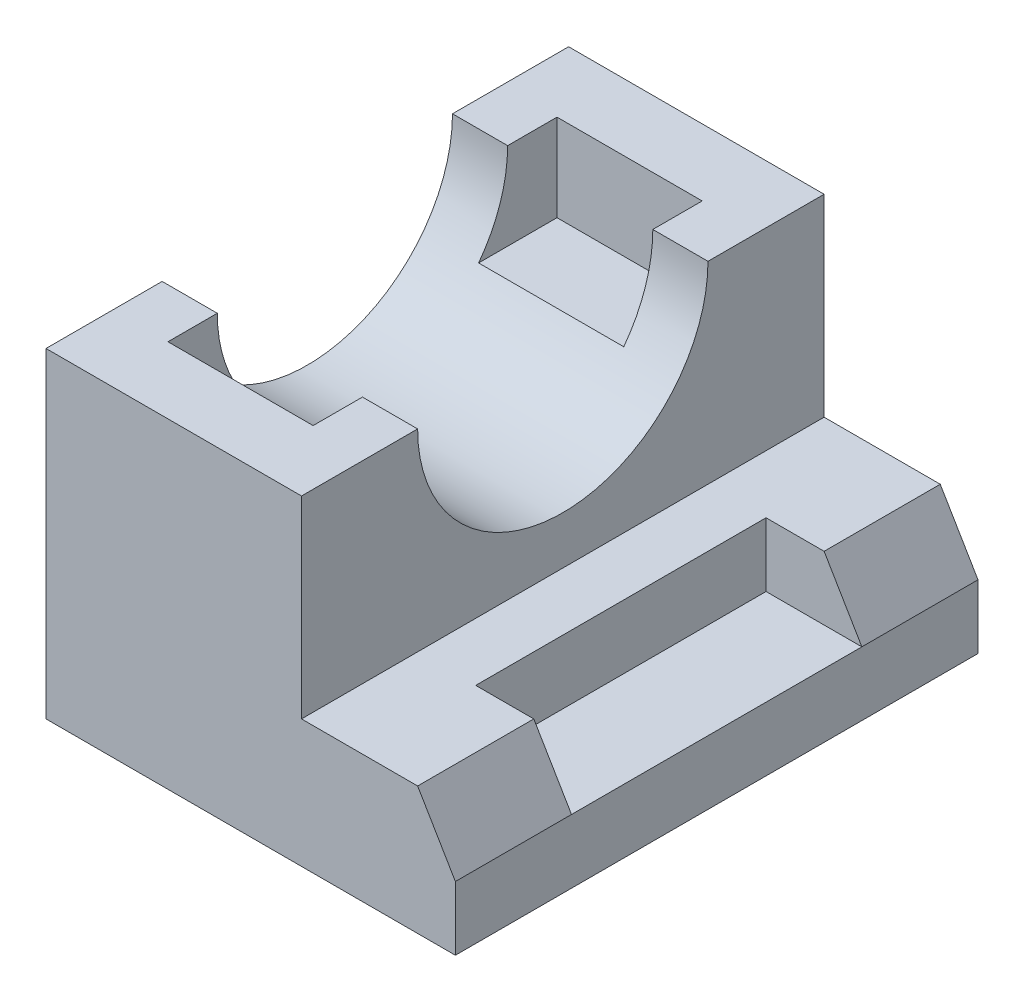
ISO-10303-21;
HEADER;
FILE_DESCRIPTION(('STEP AP214'),'2;1');
FILE_NAME('part.step','',(''),(''),'','','');
FILE_SCHEMA(('AUTOMOTIVE_DESIGN { 1 0 10303 214 1 1 1 1 }'));
ENDSEC;
DATA;
#1=APPLICATION_CONTEXT('core data for automotive mechanical design processes');
#2=APPLICATION_PROTOCOL_DEFINITION('international standard','automotive_design',2000,#1);
#3=PRODUCT_CONTEXT('',#1,'mechanical');
#4=PRODUCT('Part','Part','',(#3));
#5=PRODUCT_RELATED_PRODUCT_CATEGORY('part','',(#4));
#6=PRODUCT_DEFINITION_FORMATION('','',#4);
#7=PRODUCT_DEFINITION_CONTEXT('part definition',#1,'design');
#8=PRODUCT_DEFINITION('design','',#6,#7);
#9=PRODUCT_DEFINITION_SHAPE('','',#8);
#10=(LENGTH_UNIT() NAMED_UNIT(*) SI_UNIT(.MILLI.,.METRE.));
#11=(NAMED_UNIT(*) PLANE_ANGLE_UNIT() SI_UNIT($,.RADIAN.));
#12=(NAMED_UNIT(*) SI_UNIT($,.STERADIAN.) SOLID_ANGLE_UNIT());
#13=UNCERTAINTY_MEASURE_WITH_UNIT(LENGTH_MEASURE(1.E-05),#10,'distance_accuracy_value','');
#14=(GEOMETRIC_REPRESENTATION_CONTEXT(3) GLOBAL_UNCERTAINTY_ASSIGNED_CONTEXT((#13)) GLOBAL_UNIT_ASSIGNED_CONTEXT((#10,
#11,#12)) REPRESENTATION_CONTEXT('',''));
#15=CARTESIAN_POINT('',(0.,0.,0.));
#16=DIRECTION('',(0.,0.,1.));
#17=DIRECTION('',(1.,0.,0.));
#18=AXIS2_PLACEMENT_3D('',#15,#16,#17);
#19=CARTESIAN_POINT('',(57.0719754977029,33.7243491577335,45.));
#20=DIRECTION('',(0.860926528214316,0.50872931212664,0.));
#21=DIRECTION('',(-0.50872931212664,0.860926528214316,0.));
#22=AXIS2_PLACEMENT_3D('',#19,#20,#21);
#23=PLANE('',#22);
#24=DIRECTION('',(-0.50872931212664,0.860926528214316,0.));
#25=VECTOR('',#24,1.);
#26=CARTESIAN_POINT('',(57.071975497703,33.7243491577335,-25.));
#27=LINE('',#26,#25);
#28=CARTESIAN_POINT('',(70.5,11.,-25.));
#29=VERTEX_POINT('',#28);
#30=CARTESIAN_POINT('',(64.,22.,-25.));
#31=VERTEX_POINT('',#30);
#32=EDGE_CURVE('E251',#29,#31,#27,.T.);
#33=ORIENTED_EDGE('',*,*,#32,.F.);
#34=DIRECTION('',(0.,0.,-1.));
#35=VECTOR('',#34,1.);
#36=CARTESIAN_POINT('',(70.5,11.,45.));
#37=LINE('',#36,#35);
#38=CARTESIAN_POINT('',(70.5,11.,-45.));
#39=VERTEX_POINT('',#38);
#40=EDGE_CURVE('E312',#29,#39,#37,.T.);
#41=ORIENTED_EDGE('',*,*,#40,.T.);
#42=DIRECTION('',(0.50872931212664,-0.860926528214316,0.));
#43=VECTOR('',#42,1.);
#44=CARTESIAN_POINT('',(57.0719754977029,33.7243491577335,-45.));
#45=LINE('',#44,#43);
#46=CARTESIAN_POINT('',(64.,22.,-45.));
#47=VERTEX_POINT('',#46);
#48=EDGE_CURVE('E297',#47,#39,#45,.T.);
#49=ORIENTED_EDGE('',*,*,#48,.F.);
#50=DIRECTION('',(0.,0.,-1.));
#51=VECTOR('',#50,1.);
#52=CARTESIAN_POINT('',(64.,22.,45.));
#53=LINE('',#52,#51);
#54=EDGE_CURVE('E313',#31,#47,#53,.T.);
#55=ORIENTED_EDGE('',*,*,#54,.F.);
#56=EDGE_LOOP('',(#33,#41,#49,#55));
#57=FACE_BOUND('',#56,.T.);
#58=ADVANCED_FACE('F41',(#57),#23,.T.);
#59=CARTESIAN_POINT('',(0.,55.25,45.));
#60=DIRECTION('',(0.,-1.,0.));
#61=DIRECTION('',(1.,0.,0.));
#62=AXIS2_PLACEMENT_3D('',#59,#60,#61);
#63=PLANE('',#62);
#64=DIRECTION('',(-1.,0.,0.));
#65=VECTOR('',#64,1.);
#66=CARTESIAN_POINT('',(22.,55.25,-33.5));
#67=LINE('',#66,#65);
#68=CARTESIAN_POINT('',(34.5,55.25,-33.5));
#69=VERTEX_POINT('',#68);
#70=CARTESIAN_POINT('',(9.49999999999999,55.25,-33.5));
#71=VERTEX_POINT('',#70);
#72=EDGE_CURVE('E220',#69,#71,#67,.T.);
#73=ORIENTED_EDGE('',*,*,#72,.F.);
#74=DIRECTION('',(0.,0.,-1.));
#75=VECTOR('',#74,1.);
#76=CARTESIAN_POINT('',(34.5,55.25,-33.5));
#77=LINE('',#76,#75);
#78=CARTESIAN_POINT('',(34.5,55.25,-25.));
#79=VERTEX_POINT('',#78);
#80=EDGE_CURVE('E221',#79,#69,#77,.T.);
#81=ORIENTED_EDGE('',*,*,#80,.F.);
#82=DIRECTION('',(1.,0.,0.));
#83=VECTOR('',#82,1.);
#84=CARTESIAN_POINT('',(-1.,55.25,-25.));
#85=LINE('',#84,#83);
#86=CARTESIAN_POINT('',(44.,55.25,-25.));
#87=VERTEX_POINT('',#86);
#88=EDGE_CURVE('E256',#79,#87,#85,.T.);
#89=ORIENTED_EDGE('',*,*,#88,.T.);
#90=DIRECTION('',(0.,0.,-1.));
#91=VECTOR('',#90,1.);
#92=CARTESIAN_POINT('',(44.,55.25,45.));
#93=LINE('',#92,#91);
#94=CARTESIAN_POINT('',(44.,55.25,-45.));
#95=VERTEX_POINT('',#94);
#96=EDGE_CURVE('E286',#87,#95,#93,.T.);
#97=ORIENTED_EDGE('',*,*,#96,.T.);
#98=DIRECTION('',(-1.,0.,0.));
#99=VECTOR('',#98,1.);
#100=CARTESIAN_POINT('',(0.,55.25,-45.));
#101=LINE('',#100,#99);
#102=CARTESIAN_POINT('',(0.,55.25,-45.));
#103=VERTEX_POINT('',#102);
#104=EDGE_CURVE('E267',#95,#103,#101,.T.);
#105=ORIENTED_EDGE('',*,*,#104,.T.);
#106=DIRECTION('',(0.,0.,-1.));
#107=VECTOR('',#106,1.);
#108=CARTESIAN_POINT('',(0.,55.25,45.));
#109=LINE('',#108,#107);
#110=CARTESIAN_POINT('',(0.,55.25,-25.));
#111=VERTEX_POINT('',#110);
#112=EDGE_CURVE('E324',#111,#103,#109,.T.);
#113=ORIENTED_EDGE('',*,*,#112,.F.);
#114=CARTESIAN_POINT('',(9.49999999999999,55.25,-25.));
#115=VERTEX_POINT('',#114);
#116=EDGE_CURVE('E262',#111,#115,#85,.T.);
#117=ORIENTED_EDGE('',*,*,#116,.T.);
#118=DIRECTION('',(0.,0.,1.));
#119=VECTOR('',#118,1.);
#120=CARTESIAN_POINT('',(9.49999999999999,55.25,-18.5));
#121=LINE('',#120,#119);
#122=EDGE_CURVE('E225',#71,#115,#121,.T.);
#123=ORIENTED_EDGE('',*,*,#122,.F.);
#124=EDGE_LOOP('',(#73,#81,#89,#97,#105,#113,#117,#123));
#125=FACE_BOUND('',#124,.T.);
#126=ADVANCED_FACE('F363',(#125),#63,.F.);
#127=DIRECTION('',(1.,0.,0.));
#128=VECTOR('',#127,1.);
#129=CARTESIAN_POINT('',(22.,55.25,33.5));
#130=LINE('',#129,#128);
#131=CARTESIAN_POINT('',(9.49999999999999,55.25,33.5));
#132=VERTEX_POINT('',#131);
#133=CARTESIAN_POINT('',(34.5,55.25,33.5));
#134=VERTEX_POINT('',#133);
#135=EDGE_CURVE('E207',#132,#134,#130,.T.);
#136=ORIENTED_EDGE('',*,*,#135,.F.);
#137=DIRECTION('',(0.,0.,1.));
#138=VECTOR('',#137,1.);
#139=CARTESIAN_POINT('',(9.49999999999999,55.25,18.5));
#140=LINE('',#139,#138);
#141=CARTESIAN_POINT('',(9.49999999999999,55.25,25.));
#142=VERTEX_POINT('',#141);
#143=EDGE_CURVE('E196',#142,#132,#140,.T.);
#144=ORIENTED_EDGE('',*,*,#143,.F.);
#145=DIRECTION('',(1.,0.,0.));
#146=VECTOR('',#145,1.);
#147=CARTESIAN_POINT('',(-1.,55.25,25.));
#148=LINE('',#147,#146);
#149=CARTESIAN_POINT('',(0.,55.25,25.));
#150=VERTEX_POINT('',#149);
#151=EDGE_CURVE('E259',#150,#142,#148,.T.);
#152=ORIENTED_EDGE('',*,*,#151,.F.);
#153=CARTESIAN_POINT('',(0.,55.25,45.));
#154=VERTEX_POINT('',#153);
#155=EDGE_CURVE('E326',#154,#150,#109,.T.);
#156=ORIENTED_EDGE('',*,*,#155,.F.);
#157=DIRECTION('',(-1.,0.,0.));
#158=VECTOR('',#157,1.);
#159=CARTESIAN_POINT('',(0.,55.25,45.));
#160=LINE('',#159,#158);
#161=CARTESIAN_POINT('',(44.,55.25,45.));
#162=VERTEX_POINT('',#161);
#163=EDGE_CURVE('E269',#162,#154,#160,.T.);
#164=ORIENTED_EDGE('',*,*,#163,.F.);
#165=CARTESIAN_POINT('',(44.,55.25,25.));
#166=VERTEX_POINT('',#165);
#167=EDGE_CURVE('E308',#162,#166,#93,.T.);
#168=ORIENTED_EDGE('',*,*,#167,.T.);
#169=CARTESIAN_POINT('',(34.5,55.25,25.));
#170=VERTEX_POINT('',#169);
#171=EDGE_CURVE('E263',#170,#166,#148,.T.);
#172=ORIENTED_EDGE('',*,*,#171,.F.);
#173=DIRECTION('',(0.,0.,-1.));
#174=VECTOR('',#173,1.);
#175=CARTESIAN_POINT('',(34.5,55.25,33.5));
#176=LINE('',#175,#174);
#177=EDGE_CURVE('E195',#134,#170,#176,.T.);
#178=ORIENTED_EDGE('',*,*,#177,.F.);
#179=EDGE_LOOP('',(#136,#144,#152,#156,#164,#168,#172,#178));
#180=FACE_BOUND('',#179,.T.);
#181=ADVANCED_FACE('F43',(#180),#63,.F.);
#182=CARTESIAN_POINT('',(0.,0.,45.));
#183=DIRECTION('',(1.,0.,0.));
#184=DIRECTION('',(0.,1.,0.));
#185=AXIS2_PLACEMENT_3D('',#182,#183,#184);
#186=PLANE('',#185);
#187=ORIENTED_EDGE('',*,*,#155,.T.);
#188=CARTESIAN_POINT('',(0.,55.25,0.));
#189=DIRECTION('',(1.,0.,0.));
#190=DIRECTION('',(0.,1.,0.));
#191=AXIS2_PLACEMENT_3D('',#188,#189,#190);
#192=CIRCLE('',#191,25.);
#193=EDGE_CURVE('E265',#150,#111,#192,.T.);
#194=ORIENTED_EDGE('',*,*,#193,.T.);
#195=ORIENTED_EDGE('',*,*,#112,.T.);
#196=DIRECTION('',(0.,-1.,0.));
#197=VECTOR('',#196,1.);
#198=CARTESIAN_POINT('',(0.,0.,-45.));
#199=LINE('',#198,#197);
#200=CARTESIAN_POINT('',(0.,0.,-45.));
#201=VERTEX_POINT('',#200);
#202=EDGE_CURVE('E292',#103,#201,#199,.T.);
#203=ORIENTED_EDGE('',*,*,#202,.T.);
#204=DIRECTION('',(0.,0.,-1.));
#205=VECTOR('',#204,1.);
#206=CARTESIAN_POINT('',(0.,0.,45.));
#207=LINE('',#206,#205);
#208=CARTESIAN_POINT('',(0.,0.,45.));
#209=VERTEX_POINT('',#208);
#210=EDGE_CURVE('E325',#209,#201,#207,.T.);
#211=ORIENTED_EDGE('',*,*,#210,.F.);
#212=DIRECTION('',(0.,-1.,0.));
#213=VECTOR('',#212,1.);
#214=CARTESIAN_POINT('',(0.,0.,45.));
#215=LINE('',#214,#213);
#216=EDGE_CURVE('E272',#154,#209,#215,.T.);
#217=ORIENTED_EDGE('',*,*,#216,.F.);
#218=EDGE_LOOP('',(#187,#194,#195,#203,#211,#217));
#219=FACE_BOUND('',#218,.T.);
#220=ADVANCED_FACE('F376',(#219),#186,.F.);
#221=CARTESIAN_POINT('',(0.,0.,45.));
#222=DIRECTION('',(0.,1.,0.));
#223=DIRECTION('',(0.,0.,1.));
#224=AXIS2_PLACEMENT_3D('',#221,#222,#223);
#225=PLANE('',#224);
#226=DIRECTION('',(1.,0.,0.));
#227=VECTOR('',#226,1.);
#228=CARTESIAN_POINT('',(0.,0.,-45.));
#229=LINE('',#228,#227);
#230=CARTESIAN_POINT('',(70.5,0.,-45.));
#231=VERTEX_POINT('',#230);
#232=EDGE_CURVE('E291',#201,#231,#229,.T.);
#233=ORIENTED_EDGE('',*,*,#232,.T.);
#234=DIRECTION('',(0.,0.,-1.));
#235=VECTOR('',#234,1.);
#236=CARTESIAN_POINT('',(70.5,0.,45.));
#237=LINE('',#236,#235);
#238=CARTESIAN_POINT('',(70.5,0.,45.));
#239=VERTEX_POINT('',#238);
#240=EDGE_CURVE('E317',#239,#231,#237,.T.);
#241=ORIENTED_EDGE('',*,*,#240,.F.);
#242=DIRECTION('',(1.,0.,0.));
#243=VECTOR('',#242,1.);
#244=CARTESIAN_POINT('',(0.,0.,45.));
#245=LINE('',#244,#243);
#246=EDGE_CURVE('E277',#209,#239,#245,.T.);
#247=ORIENTED_EDGE('',*,*,#246,.F.);
#248=ORIENTED_EDGE('',*,*,#210,.T.);
#249=EDGE_LOOP('',(#233,#241,#247,#248));
#250=FACE_BOUND('',#249,.T.);
#251=ADVANCED_FACE('F384',(#250),#225,.F.);
#252=CARTESIAN_POINT('',(70.5,0.,45.));
#253=DIRECTION('',(-1.,0.,0.));
#254=DIRECTION('',(0.,0.,1.));
#255=AXIS2_PLACEMENT_3D('',#252,#253,#254);
#256=PLANE('',#255);
#257=DIRECTION('',(0.,1.,0.));
#258=VECTOR('',#257,1.);
#259=CARTESIAN_POINT('',(70.5,0.,-45.));
#260=LINE('',#259,#258);
#261=EDGE_CURVE('E293',#231,#39,#260,.T.);
#262=ORIENTED_EDGE('',*,*,#261,.T.);
#263=ORIENTED_EDGE('',*,*,#40,.F.);
#264=DIRECTION('',(0.,0.,-1.));
#265=VECTOR('',#264,1.);
#266=CARTESIAN_POINT('',(70.5,11.,-25.));
#267=LINE('',#266,#265);
#268=CARTESIAN_POINT('',(70.5,11.,25.));
#269=VERTEX_POINT('',#268);
#270=EDGE_CURVE('E241',#269,#29,#267,.T.);
#271=ORIENTED_EDGE('',*,*,#270,.F.);
#272=CARTESIAN_POINT('',(70.5,11.,45.));
#273=VERTEX_POINT('',#272);
#274=EDGE_CURVE('E316',#273,#269,#37,.T.);
#275=ORIENTED_EDGE('',*,*,#274,.F.);
#276=DIRECTION('',(0.,1.,0.));
#277=VECTOR('',#276,1.);
#278=CARTESIAN_POINT('',(70.5,0.,45.));
#279=LINE('',#278,#277);
#280=EDGE_CURVE('E279',#239,#273,#279,.T.);
#281=ORIENTED_EDGE('',*,*,#280,.F.);
#282=ORIENTED_EDGE('',*,*,#240,.T.);
#283=EDGE_LOOP('',(#262,#263,#271,#275,#281,#282));
#284=FACE_BOUND('',#283,.T.);
#285=ADVANCED_FACE('F386',(#284),#256,.F.);
#286=DIRECTION('',(0.50872931212664,-0.860926528214316,0.));
#287=VECTOR('',#286,1.);
#288=CARTESIAN_POINT('',(57.0719754977029,33.7243491577335,25.));
#289=LINE('',#288,#287);
#290=CARTESIAN_POINT('',(64.,22.,25.));
#291=VERTEX_POINT('',#290);
#292=EDGE_CURVE('E247',#291,#269,#289,.T.);
#293=ORIENTED_EDGE('',*,*,#292,.F.);
#294=CARTESIAN_POINT('',(64.,22.,45.));
#295=VERTEX_POINT('',#294);
#296=EDGE_CURVE('E315',#295,#291,#53,.T.);
#297=ORIENTED_EDGE('',*,*,#296,.F.);
#298=DIRECTION('',(0.50872931212664,-0.860926528214316,0.));
#299=VECTOR('',#298,1.);
#300=CARTESIAN_POINT('',(57.0719754977029,33.7243491577335,45.));
#301=LINE('',#300,#299);
#302=EDGE_CURVE('E278',#295,#273,#301,.T.);
#303=ORIENTED_EDGE('',*,*,#302,.T.);
#304=ORIENTED_EDGE('',*,*,#274,.T.);
#305=EDGE_LOOP('',(#293,#297,#303,#304));
#306=FACE_BOUND('',#305,.T.);
#307=ADVANCED_FACE('F408',(#306),#23,.T.);
#308=CARTESIAN_POINT('',(0.,22.,45.));
#309=DIRECTION('',(0.,1.,0.));
#310=DIRECTION('',(0.,0.,1.));
#311=AXIS2_PLACEMENT_3D('',#308,#309,#310);
#312=PLANE('',#311);
#313=DIRECTION('',(-1.,0.,0.));
#314=VECTOR('',#313,1.);
#315=CARTESIAN_POINT('',(0.,22.,-25.));
#316=LINE('',#315,#314);
#317=CARTESIAN_POINT('',(54.,22.,-25.));
#318=VERTEX_POINT('',#317);
#319=EDGE_CURVE('E328',#31,#318,#316,.T.);
#320=ORIENTED_EDGE('',*,*,#319,.F.);
#321=ORIENTED_EDGE('',*,*,#54,.T.);
#322=DIRECTION('',(1.,0.,0.));
#323=VECTOR('',#322,1.);
#324=CARTESIAN_POINT('',(0.,22.,-45.));
#325=LINE('',#324,#323);
#326=CARTESIAN_POINT('',(44.,22.,-45.));
#327=VERTEX_POINT('',#326);
#328=EDGE_CURVE('E303',#327,#47,#325,.T.);
#329=ORIENTED_EDGE('',*,*,#328,.F.);
#330=DIRECTION('',(0.,0.,-1.));
#331=VECTOR('',#330,1.);
#332=CARTESIAN_POINT('',(44.,22.,45.));
#333=LINE('',#332,#331);
#334=CARTESIAN_POINT('',(44.,22.,45.));
#335=VERTEX_POINT('',#334);
#336=EDGE_CURVE('E310',#335,#327,#333,.T.);
#337=ORIENTED_EDGE('',*,*,#336,.F.);
#338=DIRECTION('',(1.,0.,0.));
#339=VECTOR('',#338,1.);
#340=CARTESIAN_POINT('',(0.,22.,45.));
#341=LINE('',#340,#339);
#342=EDGE_CURVE('E282',#335,#295,#341,.T.);
#343=ORIENTED_EDGE('',*,*,#342,.T.);
#344=ORIENTED_EDGE('',*,*,#296,.T.);
#345=DIRECTION('',(1.,0.,0.));
#346=VECTOR('',#345,1.);
#347=CARTESIAN_POINT('',(70.5,22.,25.));
#348=LINE('',#347,#346);
#349=CARTESIAN_POINT('',(54.,22.,25.));
#350=VERTEX_POINT('',#349);
#351=EDGE_CURVE('E232',#350,#291,#348,.T.);
#352=ORIENTED_EDGE('',*,*,#351,.F.);
#353=DIRECTION('',(0.,0.,1.));
#354=VECTOR('',#353,1.);
#355=CARTESIAN_POINT('',(54.,22.,25.));
#356=LINE('',#355,#354);
#357=EDGE_CURVE('E213',#318,#350,#356,.T.);
#358=ORIENTED_EDGE('',*,*,#357,.F.);
#359=EDGE_LOOP('',(#320,#321,#329,#337,#343,#344,#352,#358));
#360=FACE_BOUND('',#359,.T.);
#361=ADVANCED_FACE('F399',(#360),#312,.T.);
#362=CARTESIAN_POINT('',(44.,0.,45.));
#363=DIRECTION('',(-1.,0.,0.));
#364=DIRECTION('',(0.,0.,1.));
#365=AXIS2_PLACEMENT_3D('',#362,#363,#364);
#366=PLANE('',#365);
#367=ORIENTED_EDGE('',*,*,#96,.F.);
#368=CARTESIAN_POINT('',(44.,55.25,0.));
#369=DIRECTION('',(1.,0.,0.));
#370=DIRECTION('',(0.,0.,-1.));
#371=AXIS2_PLACEMENT_3D('',#368,#369,#370);
#372=CIRCLE('',#371,25.);
#373=EDGE_CURVE('E254',#166,#87,#372,.T.);
#374=ORIENTED_EDGE('',*,*,#373,.F.);
#375=ORIENTED_EDGE('',*,*,#167,.F.);
#376=DIRECTION('',(0.,1.,0.));
#377=VECTOR('',#376,1.);
#378=CARTESIAN_POINT('',(44.,0.,45.));
#379=LINE('',#378,#377);
#380=EDGE_CURVE('E288',#335,#162,#379,.T.);
#381=ORIENTED_EDGE('',*,*,#380,.F.);
#382=ORIENTED_EDGE('',*,*,#336,.T.);
#383=DIRECTION('',(0.,1.,0.));
#384=VECTOR('',#383,1.);
#385=CARTESIAN_POINT('',(44.,0.,-45.));
#386=LINE('',#385,#384);
#387=EDGE_CURVE('E273',#327,#95,#386,.T.);
#388=ORIENTED_EDGE('',*,*,#387,.T.);
#389=EDGE_LOOP('',(#367,#374,#375,#381,#382,#388));
#390=FACE_BOUND('',#389,.T.);
#391=ADVANCED_FACE('F354',(#390),#366,.F.);
#392=CARTESIAN_POINT('',(0.,0.,45.));
#393=DIRECTION('',(0.,0.,1.));
#394=DIRECTION('',(1.,0.,0.));
#395=AXIS2_PLACEMENT_3D('',#392,#393,#394);
#396=PLANE('',#395);
#397=ORIENTED_EDGE('',*,*,#163,.T.);
#398=ORIENTED_EDGE('',*,*,#216,.T.);
#399=ORIENTED_EDGE('',*,*,#246,.T.);
#400=ORIENTED_EDGE('',*,*,#280,.T.);
#401=ORIENTED_EDGE('',*,*,#302,.F.);
#402=ORIENTED_EDGE('',*,*,#342,.F.);
#403=ORIENTED_EDGE('',*,*,#380,.T.);
#404=EDGE_LOOP('',(#397,#398,#399,#400,#401,#402,#403));
#405=FACE_BOUND('',#404,.T.);
#406=ADVANCED_FACE('F394',(#405),#396,.T.);
#407=CARTESIAN_POINT('',(0.,0.,-45.));
#408=DIRECTION('',(0.,0.,1.));
#409=DIRECTION('',(1.,0.,0.));
#410=AXIS2_PLACEMENT_3D('',#407,#408,#409);
#411=PLANE('',#410);
#412=ORIENTED_EDGE('',*,*,#104,.F.);
#413=ORIENTED_EDGE('',*,*,#387,.F.);
#414=ORIENTED_EDGE('',*,*,#328,.T.);
#415=ORIENTED_EDGE('',*,*,#48,.T.);
#416=ORIENTED_EDGE('',*,*,#261,.F.);
#417=ORIENTED_EDGE('',*,*,#232,.F.);
#418=ORIENTED_EDGE('',*,*,#202,.F.);
#419=EDGE_LOOP('',(#412,#413,#414,#415,#416,#417,#418));
#420=FACE_BOUND('',#419,.T.);
#421=ADVANCED_FACE('F379',(#420),#411,.F.);
#422=CARTESIAN_POINT('',(-1.,55.25,0.));
#423=DIRECTION('',(1.,0.,0.));
#424=DIRECTION('',(0.,0.,-1.));
#425=AXIS2_PLACEMENT_3D('',#422,#423,#424);
#426=CYLINDRICAL_SURFACE('',#425,25.);
#427=ORIENTED_EDGE('',*,*,#151,.T.);
#428=CARTESIAN_POINT('',(9.49999999999999,55.25,0.));
#429=DIRECTION('',(-1.,0.,0.));
#430=DIRECTION('',(0.,-1.,0.));
#431=AXIS2_PLACEMENT_3D('',#428,#429,#430);
#432=CIRCLE('',#431,25.);
#433=CARTESIAN_POINT('',(9.49999999999999,40.25,20.));
#434=VERTEX_POINT('',#433);
#435=EDGE_CURVE('E11',#142,#434,#432,.F.);
#436=ORIENTED_EDGE('',*,*,#435,.T.);
#437=DIRECTION('',(1.,0.,0.));
#438=VECTOR('',#437,1.);
#439=CARTESIAN_POINT('',(-0.999999999999993,40.25,20.));
#440=LINE('',#439,#438);
#441=CARTESIAN_POINT('',(34.5,40.25,20.));
#442=VERTEX_POINT('',#441);
#443=EDGE_CURVE('E189',#442,#434,#440,.F.);
#444=ORIENTED_EDGE('',*,*,#443,.F.);
#445=CARTESIAN_POINT('',(34.5,55.25,0.));
#446=DIRECTION('',(1.,0.,0.));
#447=DIRECTION('',(0.,1.,0.));
#448=AXIS2_PLACEMENT_3D('',#445,#446,#447);
#449=CIRCLE('',#448,25.);
#450=EDGE_CURVE('E47',#442,#170,#449,.F.);
#451=ORIENTED_EDGE('',*,*,#450,.T.);
#452=ORIENTED_EDGE('',*,*,#171,.T.);
#453=ORIENTED_EDGE('',*,*,#373,.T.);
#454=ORIENTED_EDGE('',*,*,#88,.F.);
#455=CARTESIAN_POINT('',(34.5,55.25,0.));
#456=DIRECTION('',(1.,0.,0.));
#457=DIRECTION('',(0.,1.,0.));
#458=AXIS2_PLACEMENT_3D('',#455,#456,#457);
#459=CIRCLE('',#458,25.);
#460=CARTESIAN_POINT('',(34.5,40.25,-20.));
#461=VERTEX_POINT('',#460);
#462=EDGE_CURVE('E337',#79,#461,#459,.F.);
#463=ORIENTED_EDGE('',*,*,#462,.T.);
#464=DIRECTION('',(1.,0.,0.));
#465=VECTOR('',#464,1.);
#466=CARTESIAN_POINT('',(-0.999999999999993,40.25,-20.));
#467=LINE('',#466,#465);
#468=CARTESIAN_POINT('',(9.49999999999999,40.25,-20.));
#469=VERTEX_POINT('',#468);
#470=EDGE_CURVE('E335',#461,#469,#467,.F.);
#471=ORIENTED_EDGE('',*,*,#470,.T.);
#472=CARTESIAN_POINT('',(9.49999999999999,55.25,0.));
#473=DIRECTION('',(-1.,0.,0.));
#474=DIRECTION('',(0.,-1.,0.));
#475=AXIS2_PLACEMENT_3D('',#472,#473,#474);
#476=CIRCLE('',#475,25.);
#477=EDGE_CURVE('E333',#469,#115,#476,.F.);
#478=ORIENTED_EDGE('',*,*,#477,.T.);
#479=ORIENTED_EDGE('',*,*,#116,.F.);
#480=ORIENTED_EDGE('',*,*,#193,.F.);
#481=EDGE_LOOP('',(#427,#436,#444,#451,#452,#453,#454,#463,#471,#478,#479,#480));
#482=FACE_BOUND('',#481,.T.);
#483=ADVANCED_FACE('F344',(#482),#426,.F.);
#484=CARTESIAN_POINT('',(54.,11.,-25.));
#485=DIRECTION('',(0.,0.,-1.));
#486=DIRECTION('',(-1.,0.,0.));
#487=AXIS2_PLACEMENT_3D('',#484,#485,#486);
#488=PLANE('',#487);
#489=ORIENTED_EDGE('',*,*,#32,.T.);
#490=ORIENTED_EDGE('',*,*,#319,.T.);
#491=DIRECTION('',(0.,1.,0.));
#492=VECTOR('',#491,1.);
#493=CARTESIAN_POINT('',(54.,11.,-25.));
#494=LINE('',#493,#492);
#495=CARTESIAN_POINT('',(54.,11.,-25.));
#496=VERTEX_POINT('',#495);
#497=EDGE_CURVE('E243',#496,#318,#494,.T.);
#498=ORIENTED_EDGE('',*,*,#497,.F.);
#499=DIRECTION('',(-1.,0.,0.));
#500=VECTOR('',#499,1.);
#501=CARTESIAN_POINT('',(54.,11.,-25.));
#502=LINE('',#501,#500);
#503=EDGE_CURVE('E233',#29,#496,#502,.T.);
#504=ORIENTED_EDGE('',*,*,#503,.F.);
#505=EDGE_LOOP('',(#489,#490,#498,#504));
#506=FACE_BOUND('',#505,.T.);
#507=ADVANCED_FACE('F420',(#506),#488,.F.);
#508=CARTESIAN_POINT('',(70.5,11.,25.));
#509=DIRECTION('',(0.,0.,1.));
#510=DIRECTION('',(1.,0.,0.));
#511=AXIS2_PLACEMENT_3D('',#508,#509,#510);
#512=PLANE('',#511);
#513=ORIENTED_EDGE('',*,*,#292,.T.);
#514=DIRECTION('',(1.,0.,0.));
#515=VECTOR('',#514,1.);
#516=CARTESIAN_POINT('',(70.5,11.,25.));
#517=LINE('',#516,#515);
#518=CARTESIAN_POINT('',(54.,11.,25.));
#519=VERTEX_POINT('',#518);
#520=EDGE_CURVE('E236',#519,#269,#517,.T.);
#521=ORIENTED_EDGE('',*,*,#520,.F.);
#522=DIRECTION('',(0.,1.,0.));
#523=VECTOR('',#522,1.);
#524=CARTESIAN_POINT('',(54.,11.,25.));
#525=LINE('',#524,#523);
#526=EDGE_CURVE('E246',#519,#350,#525,.T.);
#527=ORIENTED_EDGE('',*,*,#526,.T.);
#528=ORIENTED_EDGE('',*,*,#351,.T.);
#529=EDGE_LOOP('',(#513,#521,#527,#528));
#530=FACE_BOUND('',#529,.T.);
#531=ADVANCED_FACE('F415',(#530),#512,.F.);
#532=CARTESIAN_POINT('',(54.,11.,25.));
#533=DIRECTION('',(-1.,0.,0.));
#534=DIRECTION('',(0.,0.,1.));
#535=AXIS2_PLACEMENT_3D('',#532,#533,#534);
#536=PLANE('',#535);
#537=ORIENTED_EDGE('',*,*,#357,.T.);
#538=ORIENTED_EDGE('',*,*,#526,.F.);
#539=DIRECTION('',(0.,0.,1.));
#540=VECTOR('',#539,1.);
#541=CARTESIAN_POINT('',(54.,11.,25.));
#542=LINE('',#541,#540);
#543=EDGE_CURVE('E234',#496,#519,#542,.T.);
#544=ORIENTED_EDGE('',*,*,#543,.F.);
#545=ORIENTED_EDGE('',*,*,#497,.T.);
#546=EDGE_LOOP('',(#537,#538,#544,#545));
#547=FACE_BOUND('',#546,.T.);
#548=ADVANCED_FACE('F418',(#547),#536,.F.);
#549=CARTESIAN_POINT('',(0.,11.,0.));
#550=DIRECTION('',(0.,-1.,0.));
#551=DIRECTION('',(0.,0.,-1.));
#552=AXIS2_PLACEMENT_3D('',#549,#550,#551);
#553=PLANE('',#552);
#554=ORIENTED_EDGE('',*,*,#503,.T.);
#555=ORIENTED_EDGE('',*,*,#543,.T.);
#556=ORIENTED_EDGE('',*,*,#520,.T.);
#557=ORIENTED_EDGE('',*,*,#270,.T.);
#558=EDGE_LOOP('',(#554,#555,#556,#557));
#559=FACE_BOUND('',#558,.T.);
#560=ADVANCED_FACE('F411',(#559),#553,.F.);
#561=CARTESIAN_POINT('',(34.5,40.25,-33.5));
#562=DIRECTION('',(1.,0.,0.));
#563=DIRECTION('',(0.,1.,0.));
#564=AXIS2_PLACEMENT_3D('',#561,#562,#563);
#565=PLANE('',#564);
#566=ORIENTED_EDGE('',*,*,#80,.T.);
#567=DIRECTION('',(0.,1.,0.));
#568=VECTOR('',#567,1.);
#569=CARTESIAN_POINT('',(34.5,40.25,-33.5));
#570=LINE('',#569,#568);
#571=CARTESIAN_POINT('',(34.5,40.25,-33.5));
#572=VERTEX_POINT('',#571);
#573=EDGE_CURVE('E209',#572,#69,#570,.T.);
#574=ORIENTED_EDGE('',*,*,#573,.F.);
#575=DIRECTION('',(0.,0.,-1.));
#576=VECTOR('',#575,1.);
#577=CARTESIAN_POINT('',(34.5,40.25,-33.5));
#578=LINE('',#577,#576);
#579=EDGE_CURVE('E218',#461,#572,#578,.T.);
#580=ORIENTED_EDGE('',*,*,#579,.F.);
#581=ORIENTED_EDGE('',*,*,#462,.F.);
#582=EDGE_LOOP('',(#566,#574,#580,#581));
#583=FACE_BOUND('',#582,.T.);
#584=ADVANCED_FACE('F364',(#583),#565,.F.);
#585=CARTESIAN_POINT('',(9.49999999999999,40.25,-18.5));
#586=DIRECTION('',(-1.,0.,0.));
#587=DIRECTION('',(0.,-1.,0.));
#588=AXIS2_PLACEMENT_3D('',#585,#586,#587);
#589=PLANE('',#588);
#590=DIRECTION('',(0.,0.,1.));
#591=VECTOR('',#590,1.);
#592=CARTESIAN_POINT('',(9.49999999999999,40.25,-18.5));
#593=LINE('',#592,#591);
#594=CARTESIAN_POINT('',(9.49999999999999,40.25,-33.5));
#595=VERTEX_POINT('',#594);
#596=EDGE_CURVE('E63',#595,#469,#593,.T.);
#597=ORIENTED_EDGE('',*,*,#596,.F.);
#598=DIRECTION('',(0.,1.,0.));
#599=VECTOR('',#598,1.);
#600=CARTESIAN_POINT('',(9.49999999999999,40.25,-33.5));
#601=LINE('',#600,#599);
#602=EDGE_CURVE('E222',#595,#71,#601,.T.);
#603=ORIENTED_EDGE('',*,*,#602,.T.);
#604=ORIENTED_EDGE('',*,*,#122,.T.);
#605=ORIENTED_EDGE('',*,*,#477,.F.);
#606=EDGE_LOOP('',(#597,#603,#604,#605));
#607=FACE_BOUND('',#606,.T.);
#608=ADVANCED_FACE('F467',(#607),#589,.F.);
#609=CARTESIAN_POINT('',(0.,40.25,0.));
#610=DIRECTION('',(0.,-1.,0.));
#611=DIRECTION('',(1.,0.,0.));
#612=AXIS2_PLACEMENT_3D('',#609,#610,#611);
#613=PLANE('',#612);
#614=ORIENTED_EDGE('',*,*,#579,.T.);
#615=DIRECTION('',(-1.,0.,0.));
#616=VECTOR('',#615,1.);
#617=CARTESIAN_POINT('',(9.49999999999999,40.25,-33.5));
#618=LINE('',#617,#616);
#619=EDGE_CURVE('E214',#572,#595,#618,.T.);
#620=ORIENTED_EDGE('',*,*,#619,.T.);
#621=ORIENTED_EDGE('',*,*,#596,.T.);
#622=ORIENTED_EDGE('',*,*,#470,.F.);
#623=EDGE_LOOP('',(#614,#620,#621,#622));
#624=FACE_BOUND('',#623,.T.);
#625=ADVANCED_FACE('F367',(#624),#613,.F.);
#626=CARTESIAN_POINT('',(22.,40.25,-33.5));
#627=DIRECTION('',(0.,0.,-1.));
#628=DIRECTION('',(-1.,0.,0.));
#629=AXIS2_PLACEMENT_3D('',#626,#627,#628);
#630=PLANE('',#629);
#631=ORIENTED_EDGE('',*,*,#72,.T.);
#632=ORIENTED_EDGE('',*,*,#602,.F.);
#633=ORIENTED_EDGE('',*,*,#619,.F.);
#634=ORIENTED_EDGE('',*,*,#573,.T.);
#635=EDGE_LOOP('',(#631,#632,#633,#634));
#636=FACE_BOUND('',#635,.T.);
#637=ADVANCED_FACE('F369',(#636),#630,.F.);
#638=CARTESIAN_POINT('',(9.49999999999999,40.25,18.5));
#639=DIRECTION('',(-1.,0.,0.));
#640=DIRECTION('',(0.,-1.,0.));
#641=AXIS2_PLACEMENT_3D('',#638,#639,#640);
#642=PLANE('',#641);
#643=ORIENTED_EDGE('',*,*,#143,.T.);
#644=DIRECTION('',(0.,1.,0.));
#645=VECTOR('',#644,1.);
#646=CARTESIAN_POINT('',(9.49999999999999,40.25,33.5));
#647=LINE('',#646,#645);
#648=CARTESIAN_POINT('',(9.49999999999999,40.25,33.5));
#649=VERTEX_POINT('',#648);
#650=EDGE_CURVE('E192',#649,#132,#647,.T.);
#651=ORIENTED_EDGE('',*,*,#650,.F.);
#652=DIRECTION('',(0.,0.,1.));
#653=VECTOR('',#652,1.);
#654=CARTESIAN_POINT('',(9.49999999999999,40.25,18.5));
#655=LINE('',#654,#653);
#656=EDGE_CURVE('E181',#434,#649,#655,.T.);
#657=ORIENTED_EDGE('',*,*,#656,.F.);
#658=ORIENTED_EDGE('',*,*,#435,.F.);
#659=EDGE_LOOP('',(#643,#651,#657,#658));
#660=FACE_BOUND('',#659,.T.);
#661=ADVANCED_FACE('F198',(#660),#642,.F.);
#662=CARTESIAN_POINT('',(34.5,40.25,33.5));
#663=DIRECTION('',(1.,0.,0.));
#664=DIRECTION('',(0.,1.,0.));
#665=AXIS2_PLACEMENT_3D('',#662,#663,#664);
#666=PLANE('',#665);
#667=DIRECTION('',(0.,0.,-1.));
#668=VECTOR('',#667,1.);
#669=CARTESIAN_POINT('',(34.5,40.25,33.5));
#670=LINE('',#669,#668);
#671=CARTESIAN_POINT('',(34.5,40.25,33.5));
#672=VERTEX_POINT('',#671);
#673=EDGE_CURVE('E57',#672,#442,#670,.T.);
#674=ORIENTED_EDGE('',*,*,#673,.F.);
#675=DIRECTION('',(0.,1.,0.));
#676=VECTOR('',#675,1.);
#677=CARTESIAN_POINT('',(34.5,40.25,33.5));
#678=LINE('',#677,#676);
#679=EDGE_CURVE('E205',#672,#134,#678,.T.);
#680=ORIENTED_EDGE('',*,*,#679,.T.);
#681=ORIENTED_EDGE('',*,*,#177,.T.);
#682=ORIENTED_EDGE('',*,*,#450,.F.);
#683=EDGE_LOOP('',(#674,#680,#681,#682));
#684=FACE_BOUND('',#683,.T.);
#685=ADVANCED_FACE('F498',(#684),#666,.F.);
#686=CARTESIAN_POINT('',(0.,40.25,0.));
#687=DIRECTION('',(0.,1.,0.));
#688=DIRECTION('',(-1.,0.,0.));
#689=AXIS2_PLACEMENT_3D('',#686,#687,#688);
#690=PLANE('',#689);
#691=ORIENTED_EDGE('',*,*,#443,.T.);
#692=ORIENTED_EDGE('',*,*,#656,.T.);
#693=DIRECTION('',(1.,0.,0.));
#694=VECTOR('',#693,1.);
#695=CARTESIAN_POINT('',(9.49999999999999,40.25,33.5));
#696=LINE('',#695,#694);
#697=EDGE_CURVE('E190',#649,#672,#696,.T.);
#698=ORIENTED_EDGE('',*,*,#697,.T.);
#699=ORIENTED_EDGE('',*,*,#673,.T.);
#700=EDGE_LOOP('',(#691,#692,#698,#699));
#701=FACE_BOUND('',#700,.T.);
#702=ADVANCED_FACE('F183',(#701),#690,.T.);
#703=CARTESIAN_POINT('',(22.,40.25,33.5));
#704=DIRECTION('',(0.,0.,1.));
#705=DIRECTION('',(1.,0.,0.));
#706=AXIS2_PLACEMENT_3D('',#703,#704,#705);
#707=PLANE('',#706);
#708=ORIENTED_EDGE('',*,*,#135,.T.);
#709=ORIENTED_EDGE('',*,*,#679,.F.);
#710=ORIENTED_EDGE('',*,*,#697,.F.);
#711=ORIENTED_EDGE('',*,*,#650,.T.);
#712=EDGE_LOOP('',(#708,#709,#710,#711));
#713=FACE_BOUND('',#712,.T.);
#714=ADVANCED_FACE('F204',(#713),#707,.F.);
#715=CLOSED_SHELL('',(#58,#126,#181,#220,#251,#285,#307,#361,#391,#406,#421,#483,#507,#531,#548,
#560,#584,#608,#625,#637,#661,#685,#702,#714));
#716=MANIFOLD_SOLID_BREP('B2',#715);
#717=ADVANCED_BREP_SHAPE_REPRESENTATION('',(#18,#716),#14);
#718=SHAPE_DEFINITION_REPRESENTATION(#9,#717);
ENDSEC;
END-ISO-10303-21;
